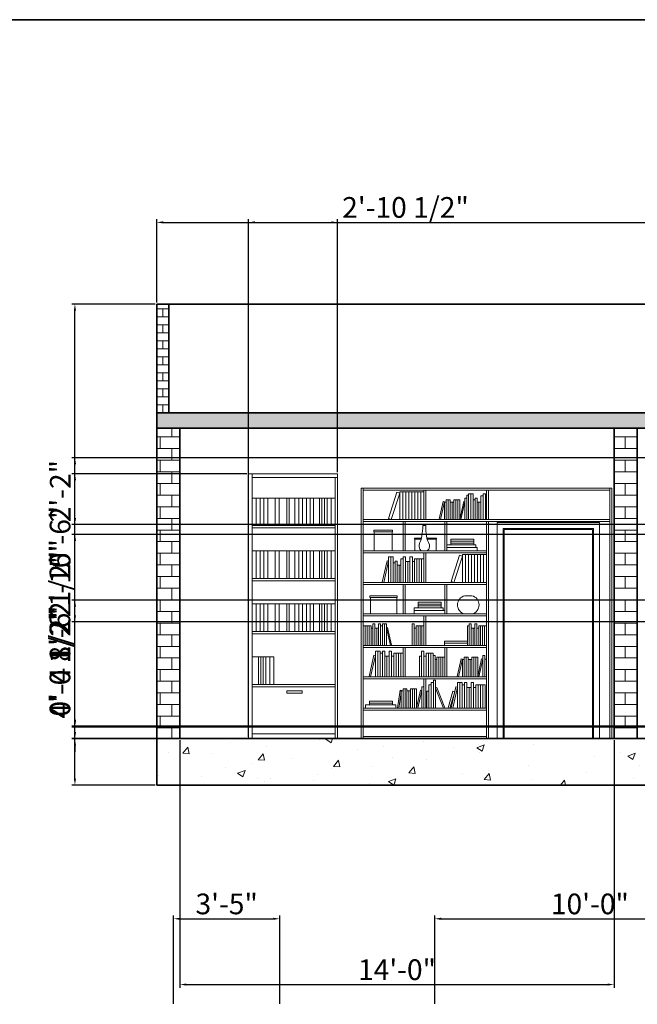
# Model space of a CAD drawing. Units: inches. Extents: x 2257 to 3678, y 834 to 1975.
# Tile 9 of 16: x 2952 to 3191, y 1594 to 1975. Entities that reach past the tile are written whole.
import ezdxf

# ---------------------------------------------------------------- set-up
doc = ezdxf.new("R2010")
doc.units = ezdxf.units.IN
for name, color, linetype, lineweight in [('A-ANNO-DIMS', 2, 'Continuous', 18), ('A-ANNO-TTLB', 7, 'Continuous', 35), ('A-FURN-ELEV', 8, 'Continuous', 13), ('A-SECT', 7, 'Continuous', 35), ('A-SECT-BRCK-PATT', 252, 'Continuous', 13), ('A-SECT-CONC-PATT', 252, 'Continuous', 13)]:
    doc.layers.add(name, color=color, linetype=linetype, lineweight=lineweight)
doc.styles.get("Standard").update_dxf_attribs({"font": 'arial.ttf'})
doc.dimstyles.new('ISO-25', dxfattribs={"dimtxt": 8, "dimasz": 2.5, "dimexe": 1.25, "dimexo": 0.625, "dimtad": 1, "dimdec": 0, "dimlunit": 3, "dimtxsty": 'Standard', "dimcen": 2.5, "dimadec": 0, "dimazin": 0, "dimtfac": 1, "dimtdec": 0, "dimtmove": 0, "dimatfit": 3, "dimfxl": 1, "dimarcsym": 0})

# ---------------------------------------------------------------- blocks, each defined once
blk = doc.blocks.new('*D62')
at = {"layer": 'A-ANNO-DIMS', "color": 0, "lineweight": -2, "transparency": 16777216}
for p, q in [((3224.23, 1485.58), (3224.23, 1669.32)), ((3218.11, 1485.58), (3225.48, 1485.58)), ((3224.23, 1443.08), (3224.23, 1483.08)), ((3218.11, 1440.58), (3225.48, 1440.58))]:
    blk.add_line(p, q, dxfattribs=at)
at = {"layer": 'A-ANNO-DIMS', "color": 0, "transparency": 16777216}
for points in [[(3223.82, 1483.08), (3224.65, 1483.08), (3224.23, 1485.58)], [(3223.82, 1443.08), (3224.65, 1443.08), (3224.23, 1440.58)]]:
    blk.add_solid(points, dxfattribs=at)
at = {"layer": 'Defpoints', "color": 0, "transparency": 16777216}
for p in [(3217.48, 1485.58), (3224.23, 1485.58), (3217.48, 1440.58)]:
    blk.add_point(p, dxfattribs=at)
at = {"layer": 'A-ANNO-DIMS', "color": 0, "transparency": 16777216, "insert": (3219.47, 1578.7), "char_height": 8, "attachment_point": 5, "rotation": 90}
blk.add_mtext('REAR BEDROOM DOOR 3\'-9" TYP.', dxfattribs=at)
blk = doc.blocks.new('*D108')
at = {"layer": 'A-ANNO-DIMS', "color": 0, "lineweight": -2, "transparency": 16777216}
for p, q in [((3011.24, 1594.2), (3011.24, 1628.38)), ((3013.74, 1627.13), (3049.79, 1627.13)), ((3052.29, 1594.2), (3052.29, 1628.38))]:
    blk.add_line(p, q, dxfattribs=at)
at = {"layer": 'A-ANNO-DIMS', "color": 0, "transparency": 16777216}
for points in [[(3013.74, 1627.54), (3013.74, 1626.71), (3011.24, 1627.13)], [(3049.79, 1627.54), (3049.79, 1626.71), (3052.29, 1627.13)]]:
    blk.add_solid(points, dxfattribs=at)
at = {"layer": 'Defpoints', "color": 0, "transparency": 16777216}
for p in [(3052.29, 1627.13), (3011.24, 1593.58), (3052.29, 1593.58)]:
    blk.add_point(p, dxfattribs=at)
at = {"layer": 'A-ANNO-DIMS', "color": 0, "transparency": 16777216, "insert": (3031.77, 1631.84), "char_height": 8, "attachment_point": 5}
blk.add_mtext('3\'-5"', dxfattribs=at)
blk = doc.blocks.new('*D109')
at = {"layer": 'A-ANNO-DIMS', "color": 0, "lineweight": -2, "transparency": 16777216}
for p, q in [((3112.29, 1594.2), (3112.29, 1628.38)), ((3114.79, 1627.13), (3229.89, 1627.13)), ((3232.39, 1594.2), (3232.39, 1628.38))]:
    blk.add_line(p, q, dxfattribs=at)
at = {"layer": 'A-ANNO-DIMS', "color": 0, "transparency": 16777216}
for points in [[(3114.79, 1627.54), (3114.79, 1626.71), (3112.29, 1627.13)], [(3229.89, 1627.54), (3229.89, 1626.71), (3232.39, 1627.13)]]:
    blk.add_solid(points, dxfattribs=at)
at = {"layer": 'Defpoints', "color": 0, "transparency": 16777216}
for p in [(3232.39, 1627.13), (3112.29, 1593.58), (3232.39, 1593.58)]:
    blk.add_point(p, dxfattribs=at)
at = {"layer": 'A-ANNO-DIMS', "color": 0, "transparency": 16777216, "insert": (3172.34, 1631.84), "char_height": 8, "attachment_point": 5}
blk.add_mtext('10\'-0"', dxfattribs=at)
blk = doc.blocks.new('*D133')
at = {"layer": 'A-ANNO-DIMS', "color": 0, "lineweight": -2, "transparency": 16777216}
for p, q in [((3004.7, 1865.47), (3004.7, 1897.74)), ((3502.7, 1865.47), (3502.7, 1897.74)), ((3007.2, 1896.49), (3500.2, 1896.49))]:
    blk.add_line(p, q, dxfattribs=at)
at = {"layer": 'A-ANNO-DIMS', "color": 0, "transparency": 16777216}
for points in [[(3007.2, 1896.91), (3007.2, 1896.07), (3004.7, 1896.49)], [(3500.2, 1896.91), (3500.2, 1896.07), (3502.7, 1896.49)]]:
    blk.add_solid(points, dxfattribs=at)
at = {"layer": 'Defpoints', "color": 0, "transparency": 16777216}
for p in [(3502.7, 1896.49), (3004.7, 1864.84), (3502.7, 1864.84)]:
    blk.add_point(p, dxfattribs=at)
at = {"layer": 'A-ANNO-DIMS', "color": 0, "transparency": 16777216, "insert": (3253.7, 1901.2), "char_height": 8, "attachment_point": 5}
blk.add_mtext('41\'-6"', dxfattribs=at)
blk = doc.blocks.new('*D134')
at = {"layer": 'A-ANNO-DIMS', "color": 0, "lineweight": -2, "transparency": 16777216}
for p, q in [((3004.08, 1864.84), (2971.8, 1864.84)), ((2973.05, 1681.34), (2973.05, 1862.34)), ((3004.08, 1678.84), (2971.8, 1678.84))]:
    blk.add_line(p, q, dxfattribs=at)
at = {"layer": 'A-ANNO-DIMS', "color": 0, "transparency": 16777216}
for points in [[(2972.63, 1862.34), (2973.47, 1862.34), (2973.05, 1864.84)], [(2972.63, 1681.34), (2973.47, 1681.34), (2973.05, 1678.84)]]:
    blk.add_solid(points, dxfattribs=at)
at = {"layer": 'Defpoints', "color": 0, "transparency": 16777216}
for p in [(2973.05, 1864.84), (3004.7, 1864.84), (3004.7, 1678.84)]:
    blk.add_point(p, dxfattribs=at)
at = {"layer": 'A-ANNO-DIMS', "color": 0, "transparency": 16777216, "insert": (2968.34, 1771.84), "char_height": 8, "attachment_point": 5, "rotation": 90}
blk.add_mtext('15\'-6"', dxfattribs=at)
blk = doc.blocks.new('*D135')
at = {"layer": 'A-ANNO-DIMS', "color": 0, "lineweight": -2, "transparency": 16777216}
for p, q in [((3013.7, 1696.22), (3013.7, 1600.44)), ((3181.7, 1696.22), (3181.7, 1600.44)), ((3016.2, 1601.69), (3179.2, 1601.69))]:
    blk.add_line(p, q, dxfattribs=at)
at = {"layer": 'A-ANNO-DIMS', "color": 0, "transparency": 16777216}
for points in [[(3016.2, 1602.1), (3016.2, 1601.27), (3013.7, 1601.69)], [(3179.2, 1602.1), (3179.2, 1601.27), (3181.7, 1601.69)]]:
    blk.add_solid(points, dxfattribs=at)
at = {"layer": 'Defpoints', "color": 0, "transparency": 16777216}
for p in [(3013.7, 1696.84), (3181.7, 1696.84), (3181.7, 1601.69)]:
    blk.add_point(p, dxfattribs=at)
at = {"layer": 'A-ANNO-DIMS', "color": 0, "transparency": 16777216, "insert": (3097.7, 1606.4), "char_height": 8, "attachment_point": 5}
blk.add_mtext('14\'-0"', dxfattribs=at)
blk = doc.blocks.new('*D141')
at = {"layer": 'A-ANNO-DIMS', "color": 0, "lineweight": -2, "transparency": 16777216}
for p, q in [((3040.22, 1697.47), (3040.22, 1897.74)), ((3074.72, 1799.88), (3074.72, 1897.74)), ((3042.72, 1896.49), (3072.22, 1896.49)), ((3074.72, 1896.49), (3124.73, 1896.49))]:
    blk.add_line(p, q, dxfattribs=at)
at = {"layer": 'A-ANNO-DIMS', "color": 0, "transparency": 16777216}
for points in [[(3042.72, 1896.91), (3042.72, 1896.07), (3040.22, 1896.49)], [(3072.22, 1896.91), (3072.22, 1896.07), (3074.72, 1896.49)]]:
    blk.add_solid(points, dxfattribs=at)
at = {"layer": 'Defpoints', "color": 0, "transparency": 16777216}
for p in [(3074.72, 1896.49), (3074.72, 1799.26), (3040.22, 1696.84)]:
    blk.add_point(p, dxfattribs=at)
at = {"layer": 'A-ANNO-DIMS', "color": 0, "transparency": 16777216, "insert": (3100.98, 1901.25), "char_height": 8, "attachment_point": 5}
blk.add_mtext('2\'-10 1/2"', dxfattribs=at)
blk = doc.blocks.new('*D142')
at = {"layer": 'A-ANNO-DIMS', "color": 0, "lineweight": -2, "transparency": 16777216}
for p, q in [((3039.59, 1799.26), (2971.8, 1799.26)), ((2973.05, 1699.34), (2973.05, 1796.76)), ((3039.59, 1696.84), (2971.8, 1696.84))]:
    blk.add_line(p, q, dxfattribs=at)
at = {"layer": 'A-ANNO-DIMS', "color": 0, "transparency": 16777216}
for points in [[(2972.63, 1796.76), (2973.47, 1796.76), (2973.05, 1799.26)], [(2972.63, 1699.34), (2973.47, 1699.34), (2973.05, 1696.84)]]:
    blk.add_solid(points, dxfattribs=at)
at = {"layer": 'Defpoints', "color": 0, "transparency": 16777216}
for p in [(2973.05, 1799.26), (3040.22, 1799.26), (3040.22, 1696.84)]:
    blk.add_point(p, dxfattribs=at)
at = {"layer": 'A-ANNO-DIMS', "color": 0, "transparency": 16777216, "insert": (2968.29, 1748.05), "char_height": 8, "attachment_point": 5, "rotation": 90}
blk.add_mtext('8\'-6 1/2"', dxfattribs=at)
blk = doc.blocks.new('*D145')
at = {"layer": 'A-ANNO-DIMS', "color": 0, "lineweight": -2, "transparency": 16777216}
for p, q in [((3353.28, 1805.46), (2971.8, 1805.46)), ((2973.05, 1782.13), (2973.05, 1802.96)), ((3353.28, 1779.63), (2971.8, 1779.63))]:
    blk.add_line(p, q, dxfattribs=at)
at = {"layer": 'A-ANNO-DIMS', "color": 0, "transparency": 16777216}
for points in [[(2972.63, 1802.96), (2973.47, 1802.96), (2973.05, 1805.46)], [(2972.63, 1782.13), (2973.47, 1782.13), (2973.05, 1779.63)]]:
    blk.add_solid(points, dxfattribs=at)
at = {"layer": 'Defpoints', "color": 0, "transparency": 16777216}
for p in [(2973.05, 1805.46), (3353.91, 1805.46), (3353.91, 1779.63)]:
    blk.add_point(p, dxfattribs=at)
at = {"layer": 'A-ANNO-DIMS', "color": 0, "transparency": 16777216, "insert": (2968.41, 1792.54), "char_height": 8, "attachment_point": 5, "rotation": 90}
blk.add_mtext('2\'-2"', dxfattribs=at)
blk = doc.blocks.new('*D146')
at = {"layer": 'A-ANNO-DIMS', "color": 0, "lineweight": -2, "transparency": 16777216}
for p, q in [((2973.05, 1703.73), (2973.05, 1747.39)), ((3353.28, 1701.23), (2971.8, 1701.23)), ((2973.05, 1696.7), (2973.05, 1701.23)), ((3353.28, 1696.7), (2971.8, 1696.7)), ((2973.05, 1694.2), (2973.05, 1691.7))]:
    blk.add_line(p, q, dxfattribs=at)
at = {"layer": 'A-ANNO-DIMS', "color": 0, "transparency": 16777216}
for points in [[(2972.63, 1703.73), (2973.47, 1703.73), (2973.05, 1701.23)], [(2972.63, 1694.2), (2973.47, 1694.2), (2973.05, 1696.7)]]:
    blk.add_solid(points, dxfattribs=at)
at = {"layer": 'Defpoints', "color": 0, "transparency": 16777216}
for p in [(2973.05, 1701.23), (3353.91, 1701.23), (3353.91, 1696.7)]:
    blk.add_point(p, dxfattribs=at)
at = {"layer": 'A-ANNO-DIMS', "color": 0, "transparency": 16777216, "insert": (2968.29, 1726.81), "char_height": 8, "attachment_point": 5, "rotation": 90}
blk.add_mtext('0\'-4 1/2"', dxfattribs=at)
blk = doc.blocks.new('*D148')
at = {"layer": 'A-ANNO-DIMS', "color": 0, "lineweight": -2, "transparency": 16777216}
for p, q in [((3375.03, 1775.78), (2971.8, 1775.78)), ((2973.05, 1744.52), (2973.05, 1773.28)), ((3375.03, 1742.02), (2971.8, 1742.02))]:
    blk.add_line(p, q, dxfattribs=at)
at = {"layer": 'A-ANNO-DIMS', "color": 0, "transparency": 16777216}
for points in [[(2972.63, 1773.28), (2973.47, 1773.28), (2973.05, 1775.78)], [(2972.63, 1744.52), (2973.47, 1744.52), (2973.05, 1742.02)]]:
    blk.add_solid(points, dxfattribs=at)
at = {"layer": 'Defpoints', "color": 0, "transparency": 16777216}
for p in [(2973.05, 1775.78), (3375.66, 1775.78), (3375.66, 1742.02)]:
    blk.add_point(p, dxfattribs=at)
at = {"layer": 'A-ANNO-DIMS', "color": 0, "transparency": 16777216, "insert": (2968.34, 1758.9), "char_height": 8, "attachment_point": 5, "rotation": 90}
blk.add_mtext('2\'-10"', dxfattribs=at)
blk = doc.blocks.new('*D149')
at = {"layer": 'A-ANNO-DIMS', "color": 0, "lineweight": -2, "transparency": 16777216}
for p, q in [((3417.18, 1750.35), (2971.8, 1750.35)), ((2973.05, 1704.19), (2973.05, 1747.85)), ((3417.18, 1701.69), (2971.8, 1701.69))]:
    blk.add_line(p, q, dxfattribs=at)
at = {"layer": 'A-ANNO-DIMS', "color": 0, "transparency": 16777216}
for points in [[(2972.63, 1747.85), (2973.47, 1747.85), (2973.05, 1750.35)], [(2972.63, 1704.19), (2973.47, 1704.19), (2973.05, 1701.69)]]:
    blk.add_solid(points, dxfattribs=at)
at = {"layer": 'Defpoints', "color": 0, "transparency": 16777216}
for p in [(2973.05, 1750.35), (3417.8, 1750.35), (3417.8, 1701.69)]:
    blk.add_point(p, dxfattribs=at)
at = {"layer": 'A-ANNO-DIMS', "color": 0, "transparency": 16777216, "insert": (2968.29, 1726.02), "char_height": 8, "attachment_point": 5, "rotation": 90}
blk.add_mtext('4\'-0 1/2"', dxfattribs=at)

msp = doc.modelspace()

# ---------------------------------------------------------------- hatches: boundary and pattern name
at = {"layer": 'A-SECT-BRCK-PATT'}
h = msp.add_hatch(dxfattribs=at)
h.set_pattern_fill('BRICK', color=256, scale=0.488189, style=0)
h.paths.add_polyline_path([(3004.7, 1822.84), (3009.45, 1822.84), (3009.45, 1864.84), (3004.7, 1864.84)])
h = msp.add_hatch(dxfattribs=at)
h.set_pattern_fill('BRICK', color=256, scale=0.708661, style=0)
h.paths.add_polyline_path([(3004.7, 1696.84), (3013.7, 1696.84), (3013.7, 1816.84), (3004.7, 1816.84)])
h = msp.add_hatch(dxfattribs=at)
h.set_pattern_fill('BRICK', color=256, scale=0.708661, style=0)
h.paths.add_polyline_path([(3181.7, 1696.84), (3190.7, 1696.84), (3190.7, 1816.84), (3181.7, 1816.84)])
at = {"layer": 'A-SECT-CONC-PATT'}
h = msp.add_hatch(dxfattribs=at)
h.set_pattern_fill('AR-CONC', color=256, scale=0.035, style=0)
h.paths.add_polyline_path([(3004.7, 1816.84), (3502.7, 1816.84), (3502.7, 1822.84), (3004.7, 1822.84)])
h = msp.add_hatch(dxfattribs=at)
h.set_pattern_fill('AR-CONC', color=256, scale=0.16, style=0)
h.paths.add_polyline_path([(3004.7, 1678.84), (3502.7, 1678.84), (3502.7, 1696.84), (3004.7, 1696.84)])

# ---------------------------------------------------------------- linework, layer by layer
at = {"layer": 'A-ANNO-TTLB'}
msp.add_lwpolyline([(2257.38, 1974.9), (3677.96, 1974.9), (3677.96, 849.42), (2257.38, 849.42)], close=True, dxfattribs=at)
at = {"layer": 'A-FURN-ELEV'}
for p, q in [((3040.22, 1799.26), (3040.22, 1696.84)), ((3040.22, 1799.26), (3040.22, 1696.84)), ((3074.72, 1799.26), (3040.22, 1799.26)), ((3074.72, 1799.26), (3040.22, 1799.26)), ((3040.22, 1797.79), (3040.22, 1698.71)), ((3041.68, 1696.84), (3041.68, 1799.26)), ((3041.68, 1797.79), (3041.68, 1779.26)), ((3073.75, 1797.79), (3041.68, 1797.79)), ((3073.75, 1779.26), (3073.75, 1797.79)), ((3074.72, 1797.79), (3074.72, 1799.26)), ((3074.72, 1779.26), (3074.72, 1797.79)), ((3041.68, 1779.26), (3073.75, 1779.26)), ((3132.33, 1696.84), (3132.33, 1780.81)), ((3133.11, 1696.84), (3133.11, 1780.81)), ((3041.68, 1778.29), (3073.75, 1778.29)), ((3041.68, 1778.29), (3041.68, 1758.78)), ((3073.75, 1758.78), (3073.75, 1778.29)), ((3074.72, 1758.78), (3074.72, 1778.29)), ((3041.68, 1758.78), (3073.75, 1758.78)), ((3041.68, 1758.78), (3073.75, 1758.78)), ((3041.68, 1758.78), (3073.75, 1758.78)), ((3041.68, 1757.8), (3073.75, 1757.8)), ((3041.68, 1757.8), (3041.68, 1738.3)), ((3073.75, 1738.3), (3073.75, 1757.8)), ((3074.72, 1738.3), (3074.72, 1757.8)), ((3041.68, 1738.3), (3073.75, 1738.3)), ((3041.68, 1738.3), (3073.75, 1738.3)), ((3041.68, 1737.32), (3073.75, 1737.32)), ((3041.68, 1737.32), (3041.68, 1717.81)), ((3041.68, 1737.32), (3073.75, 1737.32)), ((3041.68, 1737.32), (3073.75, 1737.32)), ((3073.75, 1717.81), (3073.75, 1737.32)), ((3041.68, 1717.81), (3073.75, 1717.81)), ((3132.33, 1719.94), (3084.65, 1719.94)), ((3084.65, 1719.94), (3084.65, 1697.62)), ((3041.68, 1716.84), (3073.75, 1716.84)), ((3041.68, 1716.84), (3041.68, 1698.71)), ((3073.75, 1696.84), (3073.75, 1716.84)), ((3074.72, 1696.84), (3074.72, 1716.84)), ((3132.33, 1707.77), (3084.65, 1707.77)), ((3073.75, 1698.71), (3041.68, 1698.71)), ((3188.45, 1696.84), (3076.21, 1696.84)), ((3132.33, 1696.84), (3133.11, 1696.84))]:
    msp.add_line(p, q, dxfattribs=at)
for points in [[(3040.22, 1797.79), (3040.22, 1799.26), (3074.72, 1799.26)], [(3074.72, 1799.26), (3040.22, 1799.26), (3040.22, 1696.84), (3074.72, 1696.84)], [(3040.22, 1797.79), (3040.22, 1799.26), (3074.72, 1799.26)], [(3074.72, 1797.79), (3041.68, 1797.79)], [(3074.72, 1797.79), (3041.68, 1797.79)], [(3155.78, 1792.98), (3156.56, 1792.98)], [(3180.01, 1790.67), (3180.01, 1790.67), (3180.01, 1781.58), (3179.11, 1781.58)], [(3074.72, 1789.87), (3074.72, 1779.26)], [(3176.01, 1696.84), (3176.01, 1780.42), (3136.47, 1780.42), (3136.47, 1696.84)], [(3140.66, 1781.58), (3139.5, 1781.58)], [(3141.83, 1781.58), (3140.66, 1781.58)], [(3142.99, 1781.58), (3141.83, 1781.58)], [(3144.15, 1781.58), (3142.99, 1781.58)], [(3145.32, 1781.58), (3144.15, 1781.58)], [(3146.48, 1781.58), (3145.32, 1781.58)], [(3147.64, 1781.58), (3146.48, 1781.58)], [(3148.81, 1781.58), (3147.64, 1781.58)], [(3149.97, 1781.58), (3148.81, 1781.58)], [(3151.13, 1781.58), (3149.97, 1781.58)], [(3152.29, 1781.58), (3151.13, 1781.58)], [(3153.46, 1781.58), (3152.29, 1781.58)], [(3154.62, 1781.58), (3153.46, 1781.58)], [(3155.78, 1781.58), (3154.62, 1781.58)], [(3156.56, 1781.58), (3155.78, 1781.58)], [(3170.2, 1781.58), (3169.29, 1781.58)], [(3171.11, 1781.58), (3170.2, 1781.58)], [(3172.02, 1781.58), (3171.11, 1781.58)], [(3172.93, 1781.58), (3172.02, 1781.58)], [(3173.78, 1781.58), (3172.93, 1781.58)], [(3174.63, 1781.58), (3173.78, 1781.58)], [(3175.54, 1781.58), (3174.63, 1781.58)], [(3176.4, 1781.58), (3175.54, 1781.58)], [(3177.3, 1781.58), (3176.4, 1781.58)], [(3178.2, 1781.58), (3177.3, 1781.58)], [(3179.11, 1781.58), (3178.2, 1781.58)], [(3173.69, 1696.84), (3173.69, 1778.09), (3138.8, 1778.09), (3138.8, 1696.84)], [(3173.3, 1696.84), (3173.3, 1777.71), (3139.18, 1777.71), (3139.18, 1696.84)], [(3107.09, 1773.92), (3104.44, 1773.92), (3104.44, 1774.36), (3107.21, 1774.36)], [(3107.09, 1773.92), (3104.55, 1773.92), (3104.55, 1769.41), (3112.83, 1769.41), (3112.83, 1773.92), (3109.38, 1773.92)], [(3109.26, 1774.36), (3112.94, 1774.36), (3112.94, 1773.92), (3109.38, 1773.92)], [(3074.72, 1769.39), (3074.72, 1758.78)], [(3074.72, 1717.81), (3074.71, 1717.81), (3074.71, 1728.42), (3074.72, 1728.42)], [(3074.72, 1728.42), (3074.72, 1717.81)], [(3040.22, 1698.71), (3040.22, 1696.84), (3073.75, 1696.84), (3073.75, 1698.71), (3041.68, 1698.71)], [(3074.72, 1698.71), (3074.72, 1696.84)], [(3074.72, 1698.71), (3074.72, 1696.84)]]:
    msp.add_lwpolyline(points, dxfattribs=at)
for points in [[(3041.68, 1797.79), (3041.68, 1797.79), (3041.68, 1698.71), (3041.68, 1698.71)], [(3041.68, 1779.26), (3073.75, 1779.26), (3073.75, 1797.79), (3041.68, 1797.79)], [(3074.72, 1797.79), (3073.75, 1797.79), (3073.75, 1696.84), (3074.72, 1696.84)], [(3074.72, 1797.79), (3073.75, 1797.79), (3073.75, 1696.84), (3074.72, 1696.84)], [(3084.65, 1793.75), (3083.87, 1793.75), (3083.87, 1696.84), (3084.65, 1696.84)], [(3084.65, 1793.75), (3084.65, 1792.98), (3180.01, 1792.98), (3180.01, 1793.75)], [(3097.69, 1792.15), (3098.8, 1791.79), (3095.48, 1781.58), (3094.37, 1781.94)], [(3098.8, 1792.32), (3099.96, 1792.32), (3099.96, 1781.58), (3098.8, 1781.58)], [(3099.96, 1792.32), (3101.12, 1792.32), (3101.12, 1781.58), (3099.96, 1781.58)], [(3101.12, 1792.32), (3102.29, 1792.32), (3102.29, 1781.58), (3101.12, 1781.58)], [(3102.29, 1792.32), (3103.45, 1792.32), (3103.45, 1781.58), (3102.29, 1781.58)], [(3103.45, 1792.32), (3104.61, 1792.32), (3104.61, 1781.58), (3103.45, 1781.58)], [(3104.61, 1792.32), (3105.78, 1792.32), (3105.78, 1781.58), (3104.61, 1781.58)], [(3105.78, 1792.32), (3106.94, 1792.32), (3106.94, 1781.58), (3105.78, 1781.58)], [(3106.94, 1792.32), (3108.1, 1792.32), (3108.1, 1781.58), (3106.94, 1781.58)], [(3108.88, 1792.98), (3108.1, 1792.98), (3108.1, 1781.58), (3108.88, 1781.58)], [(3125.38, 1781.58), (3124.76, 1781.58), (3124.76, 1791), (3125.38, 1791)], [(3126.29, 1781.58), (3125.38, 1781.58), (3125.38, 1791.53), (3126.29, 1791.53)], [(3127.2, 1781.58), (3126.29, 1781.58), (3126.29, 1791.53), (3127.2, 1791.53)], [(3131.03, 1781.58), (3130.13, 1781.58), (3130.13, 1790.67), (3131.03, 1790.67)], [(3131.94, 1781.58), (3131.03, 1781.58), (3131.03, 1791.53), (3131.94, 1791.53)], [(3132.33, 1792.98), (3133.11, 1792.98), (3133.11, 1781.58), (3132.33, 1781.58)], [(3180.01, 1793.75), (3180.79, 1793.75), (3180.79, 1696.84), (3180.01, 1696.84)], [(3043.18, 1789.87), (3041.68, 1789.87), (3041.68, 1779.26), (3043.18, 1779.26)], [(3044.68, 1789.87), (3043.18, 1789.87), (3043.18, 1779.26), (3044.68, 1779.26)], [(3046.18, 1789.87), (3044.68, 1789.87), (3044.68, 1779.26), (3046.18, 1779.26)], [(3047.68, 1789.87), (3046.18, 1789.87), (3046.18, 1779.26), (3047.68, 1779.26)], [(3050.6, 1789.87), (3047.68, 1789.87), (3047.68, 1779.26), (3050.6, 1779.26)], [(3050.6, 1779.26), (3052.1, 1779.26), (3052.1, 1789.87), (3050.6, 1789.87)], [(3055.02, 1789.87), (3052.1, 1789.87), (3052.1, 1779.26), (3055.02, 1779.26)], [(3055.02, 1789.87), (3055.94, 1789.87), (3055.94, 1779.26), (3055.02, 1779.26)], [(3055.94, 1789.87), (3058.15, 1789.87), (3058.15, 1779.26), (3055.94, 1779.26)], [(3059.65, 1789.87), (3058.15, 1789.87), (3058.15, 1779.26), (3059.65, 1779.26)], [(3061.15, 1789.87), (3059.65, 1789.87), (3059.65, 1779.26), (3061.15, 1779.26)], [(3062.65, 1789.87), (3061.15, 1789.87), (3061.15, 1779.26), (3062.65, 1779.26)], [(3064.15, 1789.87), (3062.65, 1789.87), (3062.65, 1779.26), (3064.15, 1779.26)], [(3064.15, 1789.87), (3065.36, 1789.87), (3065.36, 1779.26), (3064.15, 1779.26)], [(3065.36, 1779.26), (3067.74, 1779.26), (3067.74, 1789.87), (3065.36, 1789.87)], [(3067.74, 1789.87), (3068.65, 1789.87), (3068.65, 1779.26), (3067.74, 1779.26)], [(3068.65, 1779.26), (3069.63, 1779.26), (3069.63, 1789.87), (3068.65, 1789.87)], [(3069.63, 1789.87), (3070.64, 1789.87), (3070.64, 1779.26), (3069.63, 1779.26)], [(3070.64, 1779.26), (3072.17, 1779.26), (3072.17, 1789.87), (3070.64, 1789.87)], [(3072.17, 1789.87), (3073.75, 1789.87), (3073.75, 1779.26), (3072.17, 1779.26)], [(3114.56, 1781.58), (3114.07, 1781.69), (3115.6, 1788.53), (3116.1, 1788.42)], [(3116.78, 1781.58), (3116.07, 1781.58), (3116.07, 1788.28), (3116.78, 1788.28)], [(3117.53, 1781.58), (3116.78, 1781.58), (3116.78, 1789.16), (3117.53, 1789.16)], [(3118.28, 1781.58), (3117.53, 1781.58), (3117.53, 1789.16), (3118.28, 1789.16)], [(3118.99, 1781.58), (3118.28, 1781.58), (3118.28, 1788.28), (3118.99, 1788.28)], [(3119.71, 1781.58), (3118.99, 1781.58), (3118.99, 1788.28), (3119.71, 1788.28)], [(3120.46, 1781.58), (3119.71, 1781.58), (3119.71, 1789.16), (3120.46, 1789.16)], [(3121.21, 1781.58), (3120.46, 1781.58), (3120.46, 1789.16), (3121.21, 1789.16)], [(3121.97, 1781.58), (3121.21, 1781.58), (3121.21, 1789.16), (3121.97, 1789.16)], [(3122.46, 1781.58), (3121.97, 1781.69), (3123.5, 1788.53), (3124, 1788.42)], [(3124.76, 1781.58), (3124, 1781.58), (3124, 1789.87), (3124.76, 1789.87)], [(3127.95, 1781.58), (3127.2, 1781.58), (3127.2, 1789.13), (3127.95, 1789.13)], [(3128.71, 1781.58), (3127.95, 1781.58), (3127.95, 1789.85), (3128.71, 1789.85)], [(3129.42, 1781.58), (3128.71, 1781.58), (3128.71, 1788.26), (3129.42, 1788.26)], [(3130.13, 1781.58), (3129.42, 1781.58), (3129.42, 1788.26), (3130.13, 1788.26)], [(3073.75, 1778.29), (3041.68, 1778.29), (3041.68, 1779.26), (3073.75, 1779.26)], [(3073.75, 1778.29), (3041.68, 1778.29), (3041.68, 1779.26), (3073.75, 1779.26)], [(3084.65, 1781.58), (3084.65, 1780.81), (3180.01, 1780.81), (3180.01, 1781.58)], [(3100.8, 1780.81), (3100.03, 1780.81), (3100.03, 1769.41), (3100.8, 1769.41)], [(3116.95, 1780.81), (3116.18, 1780.81), (3116.18, 1769.41), (3116.95, 1769.41)], [(3073.75, 1758.78), (3041.68, 1758.78), (3041.68, 1778.29), (3073.75, 1778.29)], [(3088.67, 1776.78), (3088.67, 1777.4), (3096.01, 1777.4), (3096.01, 1776.78)], [(3095.85, 1769.41), (3088.83, 1769.41), (3088.83, 1776.78), (3095.85, 1776.78)], [(3116.95, 1770.72), (3128.17, 1770.72), (3128.17, 1771.74), (3116.95, 1771.74)], [(3118.52, 1773.19), (3127.42, 1773.19), (3127.42, 1773.91), (3118.52, 1773.91)], [(3118.52, 1772.46), (3127.42, 1772.46), (3127.42, 1773.19), (3118.52, 1773.19)], [(3118.52, 1771.74), (3127.42, 1771.74), (3127.42, 1772.46), (3118.52, 1772.46)], [(3043.18, 1769.39), (3041.68, 1769.39), (3041.68, 1758.78), (3043.18, 1758.78)], [(3044.68, 1769.39), (3043.18, 1769.39), (3043.18, 1758.78), (3044.68, 1758.78)], [(3046.18, 1769.39), (3044.68, 1769.39), (3044.68, 1758.78), (3046.18, 1758.78)], [(3047.68, 1769.39), (3046.18, 1769.39), (3046.18, 1758.78), (3047.68, 1758.78)], [(3050.6, 1769.39), (3047.68, 1769.39), (3047.68, 1758.78), (3050.6, 1758.78)], [(3050.6, 1758.78), (3052.1, 1758.78), (3052.1, 1769.39), (3050.6, 1769.39)], [(3055.02, 1769.39), (3052.1, 1769.39), (3052.1, 1758.78), (3055.02, 1758.78)], [(3055.02, 1769.39), (3055.94, 1769.39), (3055.94, 1758.78), (3055.02, 1758.78)], [(3055.94, 1769.39), (3058.15, 1769.39), (3058.15, 1758.78), (3055.94, 1758.78)], [(3059.65, 1769.39), (3058.15, 1769.39), (3058.15, 1758.78), (3059.65, 1758.78)], [(3061.15, 1769.39), (3059.65, 1769.39), (3059.65, 1758.78), (3061.15, 1758.78)], [(3062.65, 1769.39), (3061.15, 1769.39), (3061.15, 1758.78), (3062.65, 1758.78)], [(3064.15, 1769.39), (3062.65, 1769.39), (3062.65, 1758.78), (3064.15, 1758.78)], [(3064.15, 1769.39), (3065.36, 1769.39), (3065.36, 1758.78), (3064.15, 1758.78)], [(3065.36, 1758.78), (3067.74, 1758.78), (3067.74, 1769.39), (3065.36, 1769.39)], [(3067.74, 1769.39), (3068.65, 1769.39), (3068.65, 1758.78), (3067.74, 1758.78)], [(3068.65, 1758.78), (3069.63, 1758.78), (3069.63, 1769.39), (3068.65, 1769.39)], [(3068.65, 1769.39), (3069.63, 1769.39), (3069.63, 1758.78), (3068.65, 1758.78)], [(3069.63, 1769.39), (3070.64, 1769.39), (3070.64, 1758.78), (3069.63, 1758.78)], [(3070.64, 1758.78), (3072.17, 1758.78), (3072.17, 1769.39), (3070.64, 1769.39)], [(3072.17, 1769.39), (3073.75, 1769.39), (3073.75, 1758.78), (3072.17, 1758.78)], [(3084.65, 1769.41), (3084.65, 1768.63), (3132.33, 1768.63), (3132.33, 1769.41)], [(3095.36, 1757.24), (3094.45, 1757.24), (3094.45, 1767.18), (3095.36, 1767.18)], [(3096.27, 1757.24), (3095.36, 1757.24), (3095.36, 1767.18), (3096.27, 1767.18)], [(3101.02, 1757.24), (3100.11, 1757.24), (3100.11, 1767.18), (3101.02, 1767.18)], [(3103.63, 1757.24), (3102.72, 1757.24), (3102.72, 1767.18), (3103.63, 1767.18)], [(3108.88, 1768.63), (3108.1, 1768.63), (3108.1, 1757.24), (3108.88, 1757.24)], [(3116.95, 1769.41), (3128.75, 1769.41), (3128.75, 1770.72), (3116.95, 1770.72)], [(3121.92, 1767.81), (3123.03, 1767.45), (3119.71, 1757.24), (3118.6, 1757.6)], [(3123.03, 1767.97), (3124.19, 1767.97), (3124.19, 1757.24), (3123.03, 1757.24)], [(3124.19, 1767.97), (3125.35, 1767.97), (3125.35, 1757.24), (3124.19, 1757.24)], [(3125.35, 1767.97), (3126.52, 1767.97), (3126.52, 1757.24), (3125.35, 1757.24)], [(3126.52, 1767.97), (3127.68, 1767.97), (3127.68, 1757.24), (3126.52, 1757.24)], [(3127.68, 1767.97), (3128.84, 1767.97), (3128.84, 1757.24), (3127.68, 1757.24)], [(3128.84, 1767.97), (3130, 1767.97), (3130, 1757.24), (3128.84, 1757.24)], [(3130, 1767.97), (3131.17, 1767.97), (3131.17, 1757.24), (3130, 1757.24)], [(3131.17, 1767.97), (3132.33, 1767.97), (3132.33, 1757.24), (3131.17, 1757.24)], [(3092.61, 1757.24), (3092.01, 1757.37), (3093.85, 1765.58), (3094.45, 1765.45)], [(3097.02, 1757.24), (3096.27, 1757.24), (3096.27, 1764.79), (3097.02, 1764.79)], [(3097.78, 1757.24), (3097.02, 1757.24), (3097.02, 1765.5), (3097.78, 1765.5)], [(3098.49, 1757.24), (3097.78, 1757.24), (3097.78, 1763.92), (3098.49, 1763.92)], [(3099.2, 1757.24), (3098.49, 1757.24), (3098.49, 1763.92), (3099.2, 1763.92)], [(3100.11, 1757.24), (3099.2, 1757.24), (3099.2, 1766.33), (3100.11, 1766.33)], [(3101.87, 1757.24), (3101.02, 1757.24), (3101.02, 1765.28), (3101.87, 1765.28)], [(3102.72, 1757.24), (3101.87, 1757.24), (3101.87, 1765.28), (3102.72, 1765.28)], [(3104.49, 1757.24), (3103.63, 1757.24), (3103.63, 1765.28), (3104.49, 1765.28)], [(3105.39, 1757.24), (3104.49, 1757.24), (3104.49, 1766.33), (3105.39, 1766.33)], [(3106.29, 1757.24), (3105.39, 1757.24), (3105.39, 1766.33), (3106.29, 1766.33)], [(3107.2, 1757.24), (3106.29, 1757.24), (3106.29, 1766.33), (3107.2, 1766.33)], [(3108.1, 1757.24), (3107.2, 1757.24), (3107.2, 1766.33), (3108.1, 1766.33)], [(3073.75, 1757.8), (3041.68, 1757.8), (3041.68, 1758.78), (3073.75, 1758.78)], [(3073.75, 1758.78), (3041.68, 1758.78), (3041.68, 1757.8), (3073.75, 1757.8)], [(3073.75, 1757.8), (3041.68, 1757.8), (3041.68, 1738.3), (3073.75, 1738.3)], [(3084.65, 1757.24), (3084.65, 1756.46), (3132.33, 1756.46), (3132.33, 1757.24)], [(3100.8, 1756.46), (3100.03, 1756.46), (3100.03, 1745.06), (3100.8, 1745.06)], [(3116.95, 1756.46), (3116.18, 1756.46), (3116.18, 1745.06), (3116.95, 1745.06)], [(3087.24, 1751.4), (3087.24, 1752.02), (3097.76, 1752.02), (3097.76, 1751.4)], [(3043.18, 1748.91), (3041.68, 1748.91), (3041.68, 1738.3), (3043.18, 1738.3)], [(3044.68, 1748.91), (3043.18, 1748.91), (3043.18, 1738.3), (3044.68, 1738.3)], [(3046.18, 1748.91), (3044.68, 1748.91), (3044.68, 1738.3), (3046.18, 1738.3)], [(3047.68, 1748.91), (3046.18, 1748.91), (3046.18, 1738.3), (3047.68, 1738.3)], [(3050.6, 1748.91), (3047.68, 1748.91), (3047.68, 1738.3), (3050.6, 1738.3)], [(3050.6, 1738.3), (3052.1, 1738.3), (3052.1, 1748.91), (3050.6, 1748.91)], [(3055.02, 1748.91), (3052.1, 1748.91), (3052.1, 1738.3), (3055.02, 1738.3)], [(3055.02, 1748.91), (3055.94, 1748.91), (3055.94, 1738.3), (3055.02, 1738.3)], [(3055.94, 1748.91), (3058.15, 1748.91), (3058.15, 1738.3), (3055.94, 1738.3)], [(3059.65, 1748.91), (3058.15, 1748.91), (3058.15, 1738.3), (3059.65, 1738.3)], [(3061.15, 1748.91), (3059.65, 1748.91), (3059.65, 1738.3), (3061.15, 1738.3)], [(3062.65, 1748.91), (3061.15, 1748.91), (3061.15, 1738.3), (3062.65, 1738.3)], [(3064.15, 1748.91), (3062.65, 1748.91), (3062.65, 1738.3), (3064.15, 1738.3)], [(3064.15, 1748.91), (3065.36, 1748.91), (3065.36, 1738.3), (3064.15, 1738.3)], [(3065.36, 1738.3), (3067.74, 1738.3), (3067.74, 1748.91), (3065.36, 1748.91)], [(3067.74, 1748.91), (3068.65, 1748.91), (3068.65, 1738.3), (3067.74, 1738.3)], [(3068.65, 1748.91), (3069.63, 1748.91), (3069.63, 1738.3), (3068.65, 1738.3)], [(3068.65, 1738.3), (3069.63, 1738.3), (3069.63, 1748.91), (3068.65, 1748.91)], [(3069.63, 1748.91), (3070.64, 1748.91), (3070.64, 1738.3), (3069.63, 1738.3)], [(3070.64, 1738.3), (3072.17, 1738.3), (3072.17, 1748.91), (3070.64, 1748.91)], [(3072.17, 1748.91), (3073.75, 1748.91), (3073.75, 1738.3), (3072.17, 1738.3)], [(3097.6, 1745.06), (3097.6, 1751.4), (3087.39, 1751.4), (3087.39, 1745.06)], [(3105.94, 1748.84), (3114.85, 1748.84), (3114.85, 1749.56), (3105.94, 1749.56)], [(3105.94, 1748.12), (3114.85, 1748.12), (3114.85, 1748.84), (3105.94, 1748.84)], [(3105.94, 1747.4), (3114.85, 1747.4), (3114.85, 1748.12), (3105.94, 1748.12)], [(3084.65, 1745.06), (3084.65, 1744.29), (3132.33, 1744.29), (3132.33, 1745.06)], [(3104.38, 1746.37), (3115.6, 1746.37), (3115.6, 1747.4), (3104.38, 1747.4)], [(3104.38, 1745.06), (3116.18, 1745.06), (3116.18, 1746.37), (3104.38, 1746.37)], [(3108.88, 1744.29), (3108.1, 1744.29), (3108.1, 1732.89), (3108.88, 1732.89)], [(3088.37, 1732.89), (3089.13, 1732.89), (3089.13, 1741.18), (3088.37, 1741.18)], [(3090.55, 1732.89), (3091.31, 1732.89), (3091.31, 1741.18), (3090.55, 1741.18)], [(3092.06, 1732.89), (3092.82, 1732.89), (3092.82, 1741.18), (3092.06, 1741.18)], [(3092.82, 1732.89), (3093.58, 1732.89), (3093.58, 1741.18), (3092.82, 1741.18)], [(3104.38, 1732.89), (3103.62, 1732.89), (3103.62, 1741.18), (3104.38, 1741.18)], [(3126.43, 1732.89), (3125.67, 1732.89), (3125.67, 1741.16), (3126.43, 1741.16)], [(3128.61, 1732.89), (3127.85, 1732.89), (3127.85, 1741.16), (3128.61, 1741.16)], [(3073.75, 1737.32), (3041.68, 1737.32), (3041.68, 1738.3), (3073.75, 1738.3)], [(3073.75, 1717.81), (3041.68, 1717.81), (3041.68, 1737.32), (3073.75, 1737.32)], [(3084.65, 1732.89), (3085.4, 1732.89), (3085.4, 1740.47), (3084.65, 1740.47)], [(3085.4, 1732.89), (3086.16, 1732.89), (3086.16, 1740.47), (3085.4, 1740.47)], [(3086.16, 1732.89), (3086.91, 1732.89), (3086.91, 1740.47), (3086.16, 1740.47)], [(3086.91, 1732.89), (3087.66, 1732.89), (3087.66, 1740.47), (3086.91, 1740.47)], [(3087.66, 1732.89), (3088.37, 1732.89), (3088.37, 1739.59), (3087.66, 1739.59)], [(3089.13, 1732.89), (3089.84, 1732.89), (3089.84, 1739.59), (3089.13, 1739.59)], [(3089.84, 1732.89), (3090.55, 1732.89), (3090.55, 1739.59), (3089.84, 1739.59)], [(3091.31, 1732.89), (3092.06, 1732.89), (3092.06, 1740.47), (3091.31, 1740.47)], [(3095.12, 1732.89), (3095.61, 1733), (3094.08, 1739.84), (3093.58, 1739.73)], [(3105.09, 1732.89), (3104.38, 1732.89), (3104.38, 1739.59), (3105.09, 1739.59)], [(3105.84, 1732.89), (3105.09, 1732.89), (3105.09, 1740.47), (3105.84, 1740.47)], [(3106.6, 1732.89), (3105.84, 1732.89), (3105.84, 1740.47), (3106.6, 1740.47)], [(3107.35, 1732.89), (3106.6, 1732.89), (3106.6, 1740.47), (3107.35, 1740.47)], [(3108.1, 1732.89), (3107.35, 1732.89), (3107.35, 1740.47), (3108.1, 1740.47)], [(3125.67, 1732.89), (3124.92, 1732.89), (3124.92, 1740.44), (3125.67, 1740.44)], [(3127.14, 1732.89), (3126.43, 1732.89), (3126.43, 1739.57), (3127.14, 1739.57)], [(3127.85, 1732.89), (3127.14, 1732.89), (3127.14, 1739.57), (3127.85, 1739.57)], [(3129.32, 1732.89), (3128.61, 1732.89), (3128.61, 1739.57), (3129.32, 1739.57)], [(3130.07, 1732.89), (3129.32, 1732.89), (3129.32, 1740.44), (3130.07, 1740.44)], [(3130.82, 1732.89), (3130.07, 1732.89), (3130.07, 1740.44), (3130.82, 1740.44)], [(3131.58, 1732.89), (3130.82, 1732.89), (3130.82, 1740.44), (3131.58, 1740.44)], [(3132.33, 1732.89), (3131.58, 1732.89), (3131.58, 1740.44), (3132.33, 1740.44)], [(3084.65, 1732.89), (3084.65, 1732.12), (3132.33, 1732.12), (3132.33, 1732.89)], [(3116.09, 1733.68), (3124.92, 1733.68), (3124.92, 1734.48), (3116.09, 1734.48)], [(3116.09, 1732.89), (3124.92, 1732.89), (3124.92, 1733.68), (3116.09, 1733.68)], [(3087.47, 1720.72), (3086.87, 1720.85), (3088.71, 1729.06), (3089.31, 1728.93)], [(3090.22, 1720.72), (3089.31, 1720.72), (3089.31, 1730.66), (3090.22, 1730.66)], [(3091.13, 1720.72), (3090.22, 1720.72), (3090.22, 1730.66), (3091.13, 1730.66)], [(3092.03, 1720.72), (3091.13, 1720.72), (3091.13, 1729.81), (3092.03, 1729.81)], [(3092.94, 1720.72), (3092.03, 1720.72), (3092.03, 1730.66), (3092.94, 1730.66)], [(3095.56, 1720.72), (3094.65, 1720.72), (3094.65, 1730.66), (3095.56, 1730.66)], [(3097.31, 1720.72), (3096.41, 1720.72), (3096.41, 1729.81), (3097.31, 1729.81)], [(3098.22, 1720.72), (3097.31, 1720.72), (3097.31, 1729.81), (3098.22, 1729.81)], [(3099.12, 1720.72), (3098.22, 1720.72), (3098.22, 1729.81), (3099.12, 1729.81)], [(3100.03, 1720.72), (3099.12, 1720.72), (3099.12, 1729.81), (3100.03, 1729.81)], [(3100.8, 1732.12), (3100.03, 1732.12), (3100.03, 1720.72), (3100.8, 1720.72)], [(3108.13, 1720.72), (3107.22, 1720.72), (3107.22, 1730.66), (3108.13, 1730.66)], [(3109.89, 1720.72), (3108.98, 1720.72), (3108.98, 1729.81), (3109.89, 1729.81)], [(3110.79, 1720.72), (3109.89, 1720.72), (3109.89, 1729.81), (3110.79, 1729.81)], [(3111.7, 1720.72), (3110.79, 1720.72), (3110.79, 1729.81), (3111.7, 1729.81)], [(3116.95, 1732.12), (3116.18, 1732.12), (3116.18, 1720.72), (3116.95, 1720.72)], [(3041.68, 1717.81), (3044.06, 1717.81), (3044.06, 1728.42), (3041.68, 1728.42)], [(3044.06, 1728.42), (3044.97, 1728.42), (3044.97, 1717.81), (3044.06, 1717.81)], [(3044.97, 1717.81), (3045.95, 1717.81), (3045.95, 1728.42), (3044.97, 1728.42)], [(3045.95, 1728.42), (3046.96, 1728.42), (3046.96, 1717.81), (3045.95, 1717.81)], [(3046.96, 1717.81), (3048.49, 1717.81), (3048.49, 1728.42), (3046.96, 1728.42)], [(3048.49, 1728.42), (3050.07, 1728.42), (3050.07, 1717.81), (3048.49, 1717.81)], [(3093.79, 1720.72), (3092.94, 1720.72), (3092.94, 1728.76), (3093.79, 1728.76)], [(3094.65, 1720.72), (3093.79, 1720.72), (3093.79, 1728.76), (3094.65, 1728.76)], [(3096.41, 1720.72), (3095.56, 1720.72), (3095.56, 1728.76), (3096.41, 1728.76)], [(3107.22, 1720.72), (3106.37, 1720.72), (3106.37, 1728.76), (3107.22, 1728.76)], [(3108.98, 1720.72), (3108.13, 1720.72), (3108.13, 1728.76), (3108.98, 1728.76)], [(3112.45, 1720.72), (3111.7, 1720.72), (3111.7, 1729.01), (3112.45, 1729.01)], [(3113.16, 1720.72), (3112.45, 1720.72), (3112.45, 1727.42), (3113.16, 1727.42)], [(3113.92, 1720.72), (3113.16, 1720.72), (3113.16, 1728.29), (3113.92, 1728.29)], [(3114.67, 1720.72), (3113.92, 1720.72), (3113.92, 1728.29), (3114.67, 1728.29)], [(3115.42, 1720.72), (3114.67, 1720.72), (3114.67, 1728.29), (3115.42, 1728.29)], [(3116.18, 1720.72), (3115.42, 1720.72), (3115.42, 1728.29), (3116.18, 1728.29)], [(3121.52, 1720.72), (3121.02, 1720.83), (3122.56, 1727.67), (3123.05, 1727.56)], [(3123.73, 1720.72), (3123.02, 1720.72), (3123.02, 1727.42), (3123.73, 1727.42)], [(3124.48, 1720.72), (3123.73, 1720.72), (3123.73, 1728.29), (3124.48, 1728.29)], [(3125.24, 1720.72), (3124.48, 1720.72), (3124.48, 1728.29), (3125.24, 1728.29)], [(3125.95, 1720.72), (3125.24, 1720.72), (3125.24, 1727.42), (3125.95, 1727.42)], [(3126.66, 1720.72), (3125.95, 1720.72), (3125.95, 1727.42), (3126.66, 1727.42)], [(3127.41, 1720.72), (3126.66, 1720.72), (3126.66, 1728.29), (3127.41, 1728.29)], [(3128.17, 1720.72), (3127.41, 1720.72), (3127.41, 1728.29), (3128.17, 1728.29)], [(3128.92, 1720.72), (3128.17, 1720.72), (3128.17, 1728.29), (3128.92, 1728.29)], [(3129.42, 1720.72), (3128.92, 1720.83), (3130.46, 1727.67), (3130.95, 1727.56)], [(3131.71, 1720.72), (3130.95, 1720.72), (3130.95, 1729.01), (3131.71, 1729.01)], [(3132.33, 1720.72), (3131.71, 1720.72), (3131.71, 1727.56), (3132.33, 1727.56)], [(3073.75, 1716.84), (3041.68, 1716.84), (3041.68, 1717.81), (3073.75, 1717.81)], [(3073.75, 1717.81), (3041.68, 1717.81), (3041.68, 1716.84), (3073.75, 1716.84)], [(3084.65, 1720.72), (3084.65, 1719.94), (3132.33, 1719.94), (3132.33, 1720.72)], [(3108.88, 1719.94), (3108.1, 1719.94), (3108.1, 1708.55), (3108.88, 1708.55)], [(3110.86, 1708.55), (3109.96, 1708.55), (3109.96, 1717.64), (3110.86, 1717.64)], [(3111.77, 1708.55), (3110.86, 1708.55), (3110.86, 1718.49), (3111.77, 1718.49)], [(3111.77, 1719.42), (3112.55, 1719.42), (3112.55, 1708.55), (3111.77, 1708.55)], [(3121.99, 1708.55), (3121.08, 1708.55), (3121.08, 1718.49), (3121.99, 1718.49)], [(3122.9, 1708.55), (3121.99, 1708.55), (3121.99, 1718.49), (3122.9, 1718.49)], [(3123.81, 1708.55), (3122.9, 1708.55), (3122.9, 1717.64), (3123.81, 1717.64)], [(3124.72, 1708.55), (3123.81, 1708.55), (3123.81, 1718.49), (3124.72, 1718.49)], [(3127.33, 1708.55), (3126.42, 1708.55), (3126.42, 1718.49), (3127.33, 1718.49)], [(3129.09, 1708.55), (3128.19, 1708.55), (3128.19, 1717.64), (3129.09, 1717.64)], [(3129.99, 1708.55), (3129.09, 1708.55), (3129.09, 1717.64), (3129.99, 1717.64)], [(3130.9, 1708.55), (3129.99, 1708.55), (3129.99, 1717.64), (3130.9, 1717.64)], [(3131.8, 1708.55), (3130.9, 1708.55), (3130.9, 1717.64), (3131.8, 1717.64)], [(3055.05, 1715.28), (3060.93, 1715.28), (3060.93, 1714.44), (3055.05, 1714.44)], [(3098.44, 1708.55), (3097.93, 1708.62), (3098.89, 1715.56), (3099.4, 1715.49)], [(3100.05, 1708.55), (3099.34, 1708.55), (3099.34, 1715.25), (3100.05, 1715.25)], [(3100.81, 1708.55), (3100.05, 1708.55), (3100.05, 1716.12), (3100.81, 1716.12)], [(3101.56, 1708.55), (3100.81, 1708.55), (3100.81, 1716.12), (3101.56, 1716.12)], [(3102.27, 1708.55), (3101.56, 1708.55), (3101.56, 1715.25), (3102.27, 1715.25)], [(3102.98, 1708.55), (3102.27, 1708.55), (3102.27, 1715.25), (3102.98, 1715.25)], [(3103.73, 1708.55), (3102.98, 1708.55), (3102.98, 1716.12), (3103.73, 1716.12)], [(3104.49, 1708.55), (3103.73, 1708.55), (3103.73, 1716.12), (3104.49, 1716.12)], [(3105.24, 1708.55), (3104.49, 1708.55), (3104.49, 1716.12), (3105.24, 1716.12)], [(3105.74, 1708.55), (3105.24, 1708.66), (3106.78, 1715.5), (3107.27, 1715.39)], [(3108.03, 1708.55), (3107.27, 1708.55), (3107.27, 1716.83), (3108.03, 1716.83)], [(3109.96, 1708.55), (3109.25, 1708.55), (3109.25, 1715.23), (3109.96, 1715.23)], [(3115.7, 1708.55), (3116.26, 1708.78), (3113.12, 1716.58), (3112.55, 1716.35)], [(3118.13, 1708.55), (3117.45, 1708.75), (3119.35, 1715.17), (3120.03, 1714.97)], [(3119.24, 1708.55), (3118.65, 1708.68), (3120.49, 1716.89), (3121.08, 1716.76)], [(3125.57, 1708.55), (3124.72, 1708.55), (3124.72, 1716.59), (3125.57, 1716.59)], [(3126.42, 1708.55), (3125.57, 1708.55), (3125.57, 1716.59), (3126.42, 1716.59)], [(3128.19, 1708.55), (3127.33, 1708.55), (3127.33, 1716.59), (3128.19, 1716.59)], [(3087.04, 1710.58), (3095.94, 1710.58), (3095.94, 1711.3), (3087.04, 1711.3)], [(3087.04, 1709.86), (3095.94, 1709.86), (3095.94, 1710.58), (3087.04, 1710.58)], [(3084.65, 1708.55), (3084.65, 1707.77), (3132.33, 1707.77), (3132.33, 1708.55)], [(3085.48, 1708.55), (3097.27, 1708.55), (3097.27, 1709.86), (3085.48, 1709.86)], [(3084.65, 1697.62), (3084.65, 1696.84), (3132.33, 1696.84), (3132.33, 1697.62)]]:
    msp.add_lwpolyline(points, close=True, dxfattribs=at)
for points in [[(3106.56, 1772.64, 0.097042), (3107.34, 1775.12, 0.028938), (3107.68, 1779.28), (3108.79, 1779.28, 0.028938), (3109.13, 1775.12, 0.097042), (3109.91, 1772.64, -0.342723), (3109.42, 1769.41), (3107.05, 1769.41, -0.342723)], [(3123.89, 1752.04), (3126.68, 1752.04, -0.8), (3126.68, 1745.06), (3123.89, 1745.06, -0.8)]]:
    msp.add_lwpolyline(points, format="xyb", close=True, dxfattribs=at)
at = {"layer": 'A-SECT'}
for p, q in [((3004.7, 1864.84), (3004.7, 1678.84)), ((3502.7, 1864.84), (3004.7, 1864.84)), ((3009.45, 1822.84), (3009.45, 1864.84)), ((3502.7, 1822.84), (3004.7, 1822.84)), ((3009.45, 1822.84), (3009.45, 1822.84)), ((3196.31, 1816.84), (3004.7, 1816.84)), ((3013.7, 1816.84), (3013.7, 1696.84)), ((3181.7, 1696.84), (3181.7, 1816.84)), ((3190.7, 1696.84), (3190.7, 1816.84)), ((3502.7, 1696.84), (3004.7, 1696.84)), ((3502.7, 1678.84), (3004.7, 1678.84))]:
    msp.add_line(p, q, dxfattribs=at)

# ---------------------------------------------------------------- dimensions: what is measured, and where the dimension line sits
at = {"layer": 'A-ANNO-DIMS'}
for base, p1, p2, picture, middle in [((3074.72, 1896.49), (3040.22, 1696.84), (3074.72, 1799.26), '*D141', (3100.98, 1901.25)), ((3502.7, 1896.49), (3004.7, 1864.84), (3502.7, 1864.84), '*D133', (3253.7, 1901.2)), ((3181.7, 1601.69), (3013.7, 1696.84), (3181.7, 1696.84), '*D135', (3097.7, 1606.4)), ((3052.2934, 1627.1269), (3011.2405, 1593.5769), (3052.2934, 1593.5769), '*D108', (3031.7669, 1631.8393)), ((3232.39, 1627.13), (3112.29, 1593.58), (3232.39, 1593.58), '*D109', (3172.34, 1631.84))]:
    dim = msp.add_linear_dim(base=base, p1=p1, p2=p2, dimstyle='ISO-25', override={"dimdec": 1, "dimlfac": 1, "dimrnd": 0, "dimzin": 1, "dimdsep": 46, "dimlunit": 4, "dimfrac": 2}, dxfattribs=at)
    dim.commit()
    dim.dimension.update_dxf_attribs({"geometry": picture, "text_midpoint": middle})
for base, p1, p2, picture, middle in [((2973.05, 1864.84), (3004.7, 1678.84), (3004.7, 1864.84), '*D134', (2968.34, 1771.84)), ((2973.05, 1805.46), (3353.91, 1779.63), (3353.91, 1805.46), '*D145', (2968.41, 1792.54)), ((2973.05, 1799.26), (3040.22, 1696.84), (3040.22, 1799.26), '*D142', (2968.29, 1748.05)), ((2973.05, 1775.78), (3375.66, 1742.02), (3375.66, 1775.78), '*D148', (2968.34, 1758.9)), ((2973.05, 1750.35), (3417.8, 1701.69), (3417.8, 1750.35), '*D149', (2968.29, 1726.02)), ((2973.05, 1701.23), (3353.91, 1696.7), (3353.91, 1701.23), '*D146', (2968.29, 1726.81))]:
    dim = msp.add_linear_dim(base=base, p1=p1, p2=p2, angle=90, dimstyle='ISO-25', override={"dimdec": 1, "dimlfac": 1, "dimrnd": 0, "dimzin": 1, "dimdsep": 46, "dimlunit": 4, "dimfrac": 2}, dxfattribs=at)
    dim.commit()
    dim.dimension.update_dxf_attribs({"geometry": picture, "text_midpoint": middle})
dim = msp.add_linear_dim(base=(3224.23, 1485.58), p1=(3217.48, 1440.58), p2=(3217.48, 1485.58), angle=90, text='REAR BEDROOM DOOR <> TYP.', dimstyle='ISO-25', override={"dimdec": 1, "dimlfac": 1, "dimrnd": 0, "dimzin": 1, "dimdsep": 46, "dimlunit": 4, "dimfrac": 2}, dxfattribs=at)
dim.commit()
dim.dimension.update_dxf_attribs({"geometry": '*D62', "text_midpoint": (3219.47, 1578.7)})

doc.saveas('drawing.dxf')
